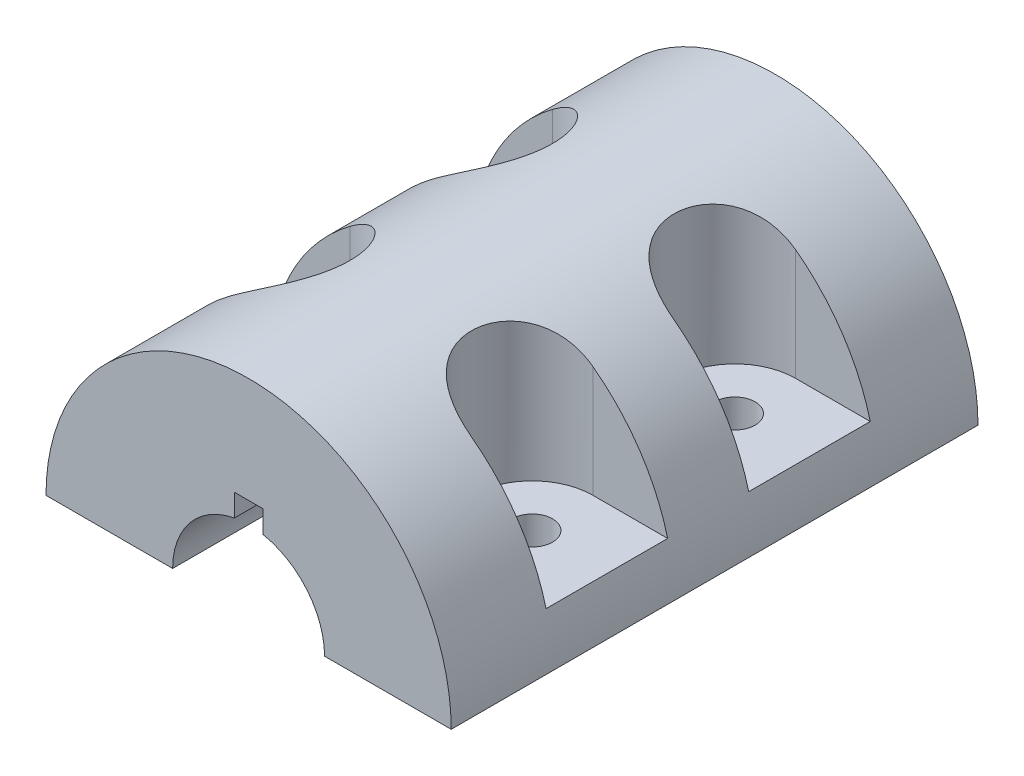
SolidWorks part; units mm, degrees
material "Plain Carbon Steel"
ref_plane "Front Plane" through (0, 0, 0) normal (0, 0, 1) x (1, 0, 0)
ref_plane "Top Plane" through (0, 0, 0) normal (0, 1, 0) x (1, 0, 0)
ref_plane "Right Plane" through (0, 0, 0) normal (1, 0, 0) x (0, 0, -1)
sketch "Housing Profile Sketch" plane through (0, 0, 0) normal (0, 0, 1) x (1, 0, 0)
  line L0 (-100, 0) -> (-37.5, 0)
  line L1 (37.5, 0) -> (100, 0)
  arc A0 (100, 0) -> (-100, 0) centre (0, 0) ccw
  arc A1 (37.5, 0) -> (-37.5, 0) centre (0, 0) ccw
  dimension "D1" = 200
  dimension "D2" = 75
extrude "Housing Body" add sketch "Housing Profile Sketch" along normal mid plane 260
sketch "Bolt Pocket Sketch" plane through (0, 0, 0) normal (0, 1, 0) x (1, 0, 0)
  line L0 (-60, -20) -> (-100, -20)
  line L1 (-100, -20) -> (-100, -80)
  line L2 (-100, -80) -> (-60, -80)
  line L3 (-100, -130) -> (100, -130) construction
  line L4 (-100, -130) -> (-100, 130) construction
  arc A0 (-60, -80) -> (-60, -20) centre (-60, -50) ccw
  dimension "D1" = 60
  dimension "D2" = 80
  dimension "D4" = 40
extrude "Bolt Pocket" cut sketch "Bolt Pocket Sketch" along normal blind 260 from offset 25
mirror "Bolt Pocket Mirror Front" about plane through (0, 0, 0) normal (0, 0, 1) of "Bolt Pocket"
mirror "Bolt Pocket Mirror Right" about plane through (0, 0, 0) normal (1, 0, 0) of "Bolt Pocket Mirror Front", "Bolt Pocket"
sketch "Bolt Hole Sketch" plane through (0, 25, 0) normal (0, 1, 0) x (1, 0, 0)
  line L0 (-60, -80) -> (-60, -20) construction
  circle A0 centre (-60, -50) radius 10
  arc A1 (-60, -80) -> (-60, -20) centre (-60, -50) ccw construction
  dimension "D1" = 20
extrude "Bolt Hole Ø20" cut sketch "Bolt Hole Sketch" against normal blind 260
mirror "Bolt Hole Mirror Front" about plane through (0, 0, 0) normal (0, 0, 1) of "Bolt Hole Ø20"
mirror "Bolt Hole Mirror Right" about plane through (0, 0, 0) normal (1, 0, 0) of "Bolt Hole Mirror Front", "Bolt Hole Ø20"
sketch "Notch Sketch" plane through (0, 0, -130) normal (0, 0, -1) x (-1, 0, 0)
  line L0 (0, 0) -> (0, 121.9621) construction
  line L2 (-7, 47.8409) -> (7, 47.8409)
  line L3 (-7, 47.8409) -> (-7, 36.8409)
  line L5 (7, 47.8409) -> (7, 36.8409)
  line L6 (-7, 47.8409) -> (7, 36.8409) construction
  line L7 (-7, 36.8409) -> (7, 47.8409) construction
  arc A0 (37.5, 0) -> (-37.5, 0) centre (0, 0) ccw construction
  arc A1 (7, 36.8409) -> (-7, 36.8409) centre (0, 0) ccw
  point P3 (0, 42.3409)
  dimension "D1" = 14
  dimension "D2" = 11
extrude "Notch Cut" cut sketch "Notch Sketch" against normal through all
